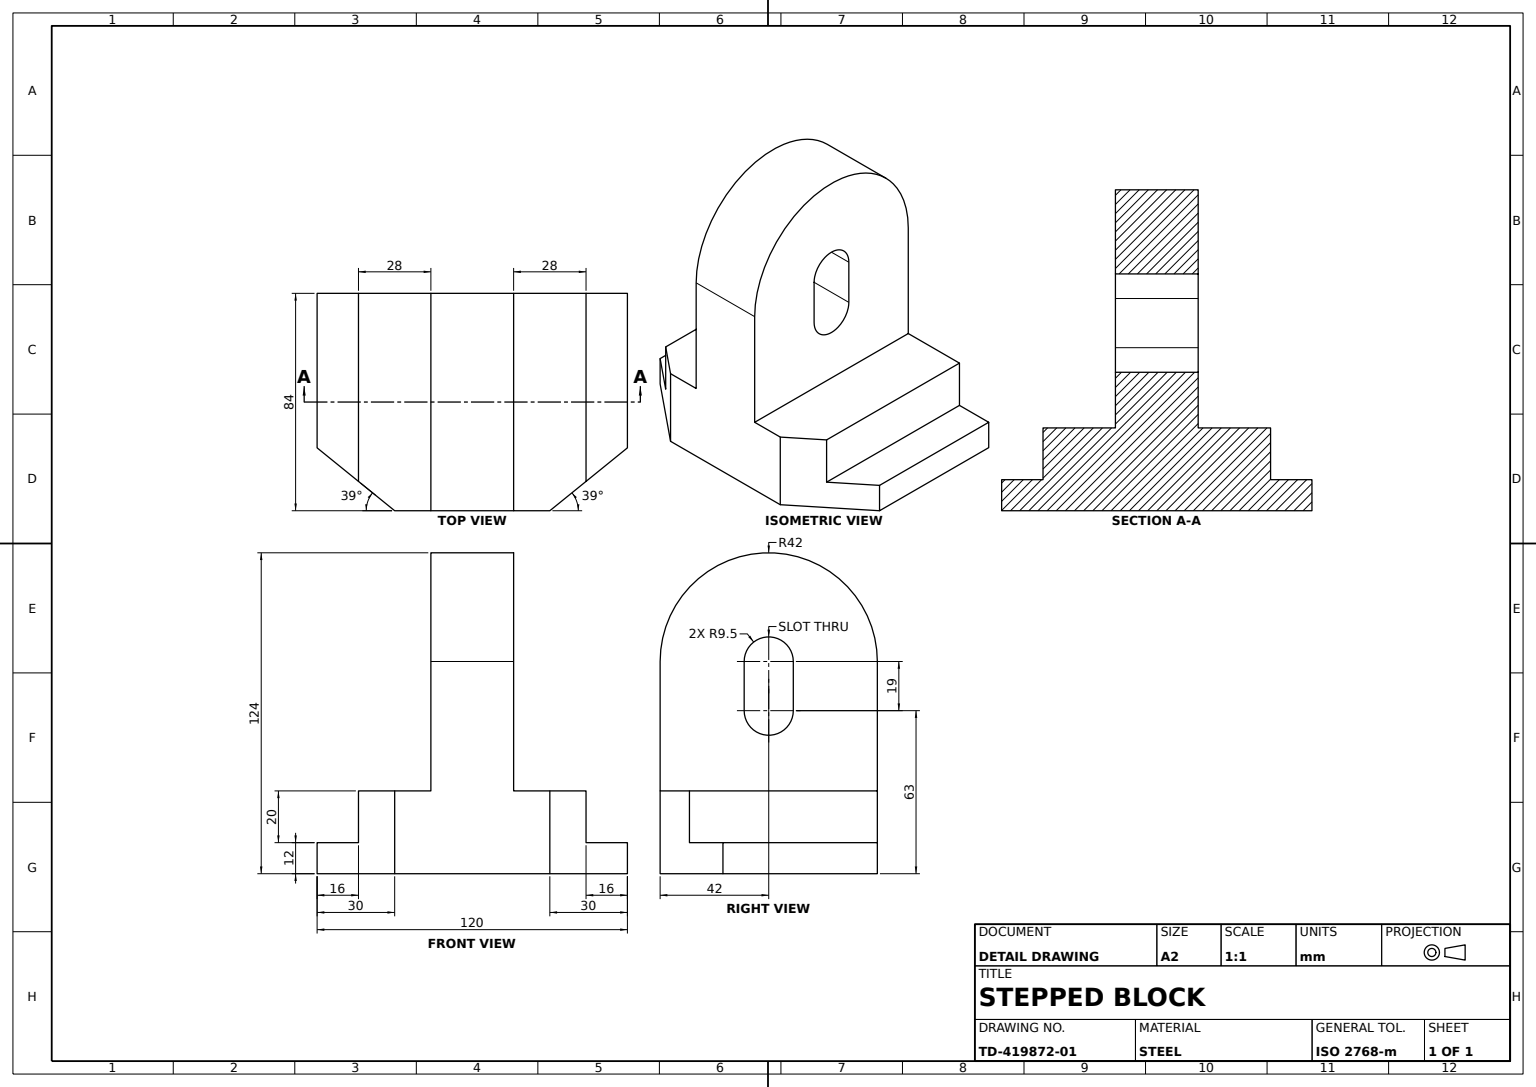
from build123d import *

# Parameters (mm, degrees)
BRACKET_BODY_DEPTH            = 42
UPRIGHT_PROFILE_CUT_DEPTH     = 40
GUIDE_SLOT_DEPTH              = 40
ANGLED_CORNER_CUT_39DEG_DEPTH = 40


with BuildPart() as part:
    # Bracket Side Profile Sketch → Bracket Body (new, symmetric)
    with BuildSketch(Plane(origin=(0, 0, 0), x_dir=(0, 0, -1), z_dir=(1, 0, 0))):
        Polygon((-60, 0), (60, 0), (60, 12), (44, 12), (44, 32), (16, 32), (16, 124), (-16, 124), (-16, 32), (-44, 32), (-44, 12), (-60, 12), align=None)
    extrude(amount=BRACKET_BODY_DEPTH, both=True)

    # Upright Profile Cut Sketch → Upright Profile Cut (cut)
    with BuildSketch(Plane(origin=(0, 0, -16), x_dir=(-1, 0, 0), z_dir=(0, 0, -1))):
        with BuildLine():
            Line((-42, 124), (-42, 82))
            ThreePointArc((-42, 82), (-29.69848481, 111.69848481), (0, 124))
            Line((0, 124), (-42, 124))
        make_face()
        with BuildLine():
            Line((42, 124), (0, 124))
            ThreePointArc((0, 124), (29.69848481, 111.69848481), (42, 82))
            Line((42, 82), (42, 124))
        make_face()
    extrude(amount=-UPRIGHT_PROFILE_CUT_DEPTH, mode=Mode.SUBTRACT)

    # Guide Slot Sketch → Guide Slot (cut)
    with BuildSketch(Plane(origin=(0, 0, -16), x_dir=(-1, 0, 0), z_dir=(0, 0, -1))):
        with BuildLine():
            Line((9.5, 82), (9.5, 63))
            ThreePointArc((9.5, 63), (0, 53.5), (-9.5, 63))
            Line((-9.5, 63), (-9.5, 82))
            ThreePointArc((-9.5, 82), (0, 91.5), (9.5, 82))
        make_face()
    extrude(amount=-GUIDE_SLOT_DEPTH, mode=Mode.SUBTRACT)

    # Angled Corner Cut Sketch 39deg → Angled Corner Cut 39deg (cut)
    with BuildSketch(Plane(origin=(0, 32, 0), x_dir=(1, 0, 0), z_dir=(0, 1, 0))):
        Polygon((42, 30), (17.706479004, 60), (42, 60), align=None)
        Polygon((42, -60), (42, -30), (17.706479004, -60), align=None)
    extrude(amount=-ANGLED_CORNER_CUT_39DEG_DEPTH, mode=Mode.SUBTRACT)


solid = part.part
